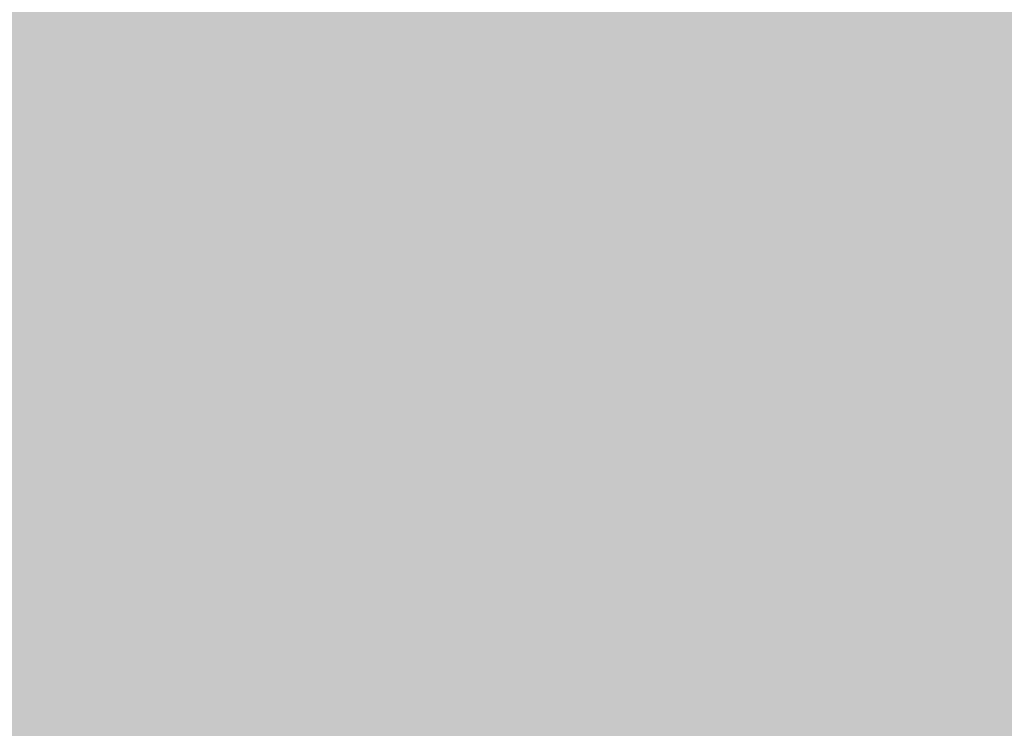
# Model space of a CAD drawing. Units: feet. Extents: x 3168 to 4724, y 827 to 1477.
# Tile 122 of 256: x 3298.685 to 3303.032, y 1093.654 to 1096.781. Entities that reach past the tile are written whole.
import ezdxf

# ---------------------------------------------------------------- set-up
doc = ezdxf.new("R2010")
doc.units = ezdxf.units.FT
doc.layers.add('A-ELEV-PATT', color=8, linetype='Continuous', lineweight=13)

msp = doc.modelspace()

# ---------------------------------------------------------------- hatches: boundary and pattern name
at = {"layer": 'A-ELEV-PATT'}
h = msp.add_hatch(color=256, dxfattribs=at)
h.dxf.hatch_style = 1
edge = h.paths.add_edge_path()
edge.add_ellipse((3552.9058, 979.2201), major_axis=(36.7449, 0), ratio=0.4848485, start_angle=0, end_angle=360)
edge = h.paths.add_edge_path()
edge.add_ellipse((3559.8916, 929.2523), major_axis=(36.7449, 0), ratio=0.4848485, start_angle=0, end_angle=360)
edge = h.paths.add_edge_path()
edge.add_line((3299.3168, 1198.6061), (3479.9167, 1198.6061))
edge.add_line((3479.9167, 1198.6061), (3479.9167, 1209.8686))
edge.add_spline(control_points=[(3479.9167, 1209.8686), (3464.3012, 1209.8686), (3448.6856, 1209.8686), (3410.9491, 1209.8686), (3388.8282, 1209.8686), (3355.6469, 1209.8686), (3344.5864, 1209.8686), (3327.9957, 1209.8686), (3322.4655, 1209.8686), (3314.1702, 1209.8686), (3311.4051, 1209.8686), (3307.2574, 1209.8686), (3305.8748, 1209.8686), (3303.801, 1209.8686), (3303.1097, 1209.8686), (3302.0728, 1209.8686), (3301.7272, 1209.8686), (3301.2087, 1209.8686), (3301.0359, 1209.8686), (3300.7767, 1209.8686), (3300.6903, 1209.8686), (3300.5606, 1209.8686), (3300.5174, 1209.8686), (3300.4526, 1209.8686), (3300.431, 1209.8686), (3300.3986, 1209.8686), (3300.3878, 1209.8686), (3300.3662, 1209.8686), (3300.3457, 1209.8686), (3300.3455, 1209.8686), (3300.3455, 1209.8686), (3300.3433, 1209.8686), (3300.3411, 1209.8686), (3300.3379, 1209.8686), (3300.3368, 1209.8686), (3300.3339, 1209.8686), (3300.3321, 1209.8686), (3300.3255, 1209.8686), (3300.3207, 1209.8686), (3300.3109, 1209.8686), (3300.306, 1209.8686), (3300.2905, 1209.8686), (3300.28, 1209.8686), (3300.2324, 1209.8688), (3300.1953, 1209.869), (3299.9511, 1209.8706), (3299.7448, 1209.8743), (3299.4368, 1209.8833), (3299.3344, 1209.8868), (3299.1811, 1209.8929), (3299.13, 1209.8951), (3298.6522, 1209.9168), (3298.2295, 1209.9457), (3297.6016, 1210.0024), (3297.3934, 1210.0235), (3297.0827, 1210.0583), (3296.9793, 1210.0705), (3296.293, 1210.1549), (3295.7181, 1210.2434), (3294.8687, 1210.3989), (3294.5877, 1210.4545), (3294.1693, 1210.5433), (3294.0304, 1210.5739), (3291.7071, 1211.1012), (3289.6536, 1211.8134), (3285.7763, 1213.564), (3283.9514, 1214.6035), (3280.5122, 1216.9801), (3278.8972, 1218.3176), (3276.3799, 1220.8295), (3275.416, 1221.9177), (3274.0393, 1223.7077), (3273.581, 1224.3495), (3273.1432, 1225.0163)], knot_values=[39.119033, 39.119033, 39.119033, 39.119033, 39.286353, 39.286353, 39.523379, 39.523379, 39.641892, 39.641892, 39.701148, 39.701148, 39.730777, 39.730777, 39.745591, 39.745591, 39.752998, 39.752998, 39.756701, 39.756701, 39.758553, 39.758553, 39.759479, 39.759479, 39.759942, 39.759942, 39.760173, 39.760173, 39.760289, 39.760289, 39.760405, 39.760405, 39.760463, 39.760463, 39.763389, 39.763389, 39.764851, 39.764851, 39.767304, 39.767304, 39.773825, 39.773825, 39.78057, 39.78057, 39.79477, 39.79477, 39.845194, 39.845194, 40.126715, 40.126715, 40.267476, 40.267476, 40.337856, 40.337856, 40.927023, 40.927023, 41.221606, 41.221606, 41.368898, 41.368898, 42.202622, 42.202622, 42.619485, 42.619485, 42.827916, 42.827916, 46.118323, 46.118323, 49.408731, 49.408731, 52.699139, 52.699139, 54.927489, 54.927489, 56.104228, 56.104228, 56.104228, 56.104228], weights=[1, 1, 1, 1, 1, 1, 1, 1, 1, 1, 1, 1, 1, 1, 1, 1, 1, 1, 1, 1, 1, 1, 1, 1, 1, 1, 1, 1, 1, 1, 1, 1, 1, 1, 1, 1, 1, 1, 1, 1, 1, 1, 1, 1, 1, 1, 1, 1, 1, 1, 1, 1, 1, 1, 1, 1, 1, 1, 1, 1, 1, 1, 1, 1, 1, 1, 1, 1, 1, 1, 1, 1, 1, 1], degree=3, periodic=0)
edge.add_line((3273.1432, 1225.0163), (3273.1432, 1099.0163))
edge.add_line((3273.1432, 1099.0163), (3299.3168, 1099.0163))
edge.add_line((3299.3168, 1099.0163), (3299.3168, 1198.6061))
edge = h.paths.add_edge_path()
edge.add_line((3304.7584, 1324.1581), (3479.9167, 1324.1581))
edge.add_line((3479.9167, 1324.1581), (3479.9167, 1335.7146))
edge.add_line((3479.9167, 1335.7146), (3269.1616, 1335.7146))
edge.add_spline(control_points=[(3269.1616, 1335.7146), (3264.0242, 1335.7146), (3258.3641, 1328.9582), (3259.2643, 1323.9003)], knot_values=[0, 0, 0, 0, 15.412191, 15.412191, 15.412191, 15.412191], degree=3, periodic=0)
edge.add_line((3259.2643, 1323.9003), (3265.5168, 1288.7691))
edge.add_line((3265.5168, 1288.7691), (3275.2651, 1261.5456))
edge.add_line((3275.2651, 1261.5456), (3304.7584, 1261.5456))
edge.add_line((3304.7584, 1261.5456), (3304.7584, 1324.1581))
h = msp.add_hatch(color=256, dxfattribs=at)
h.dxf.hatch_style = 1
h.paths.add_polyline_path([(3384.5252, 1099.0163), (3335.0292, 1099.0163), (3299.3168, 1099.0163), (3273.1432, 1099.0163), (3217.5654, 1099.0163), (3168.0693, 827.1163), (3335.0292, 827.1163)])

doc.saveas('drawing.dxf')
